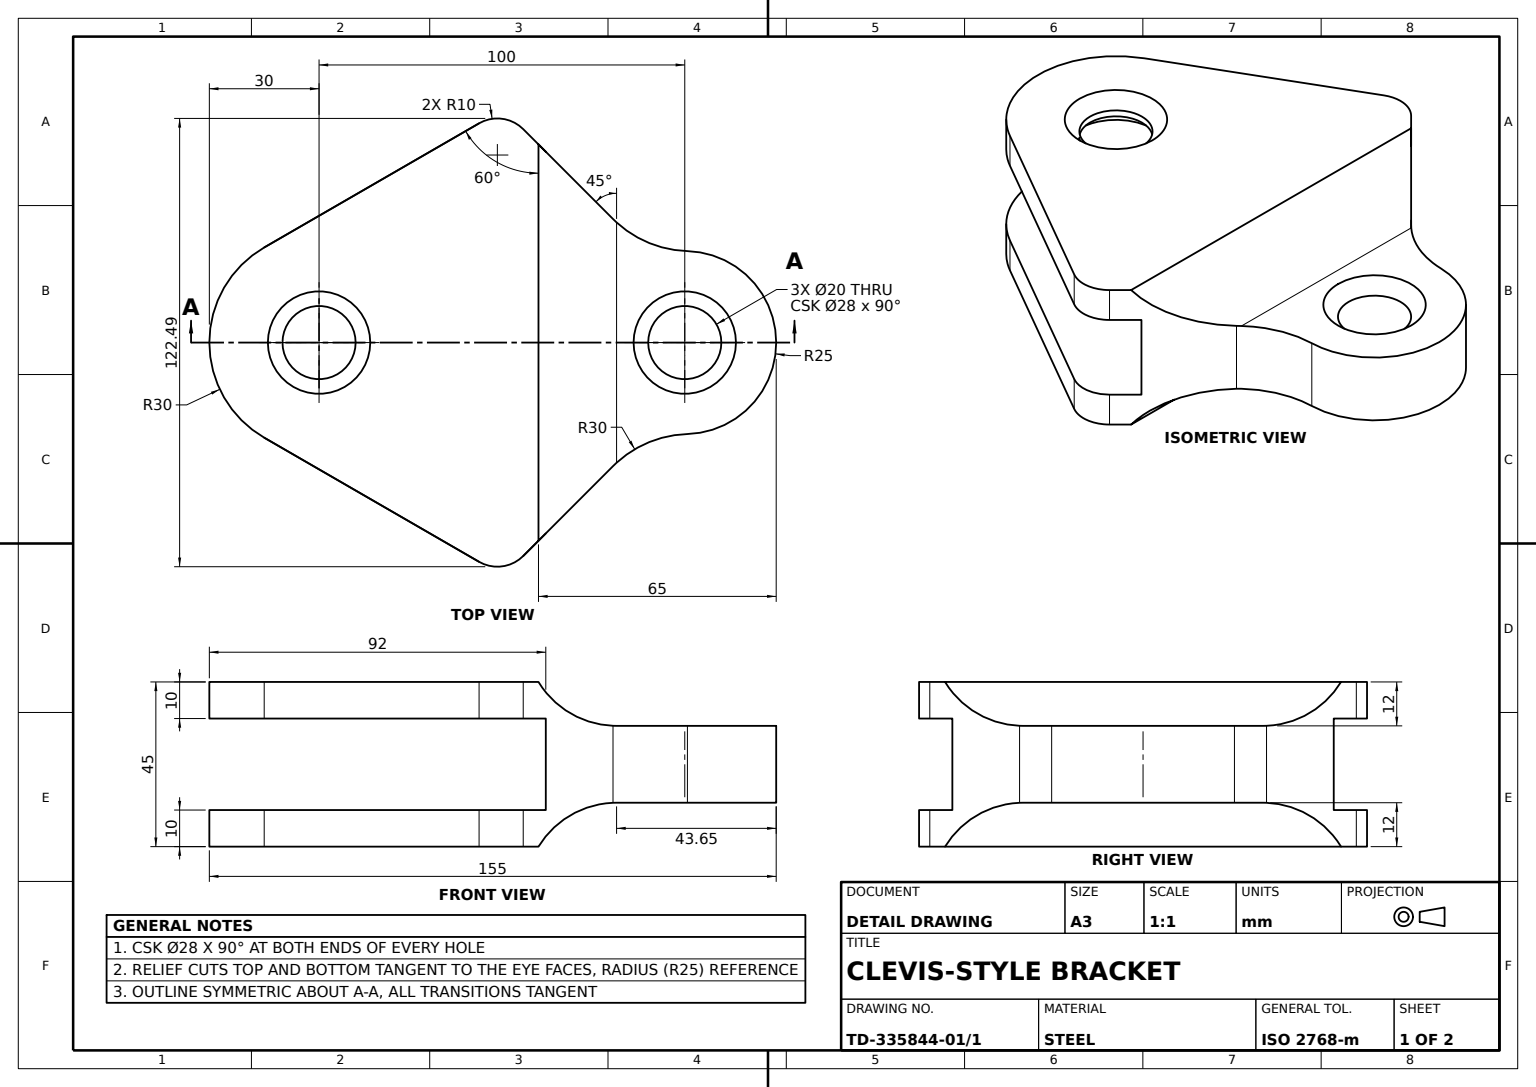
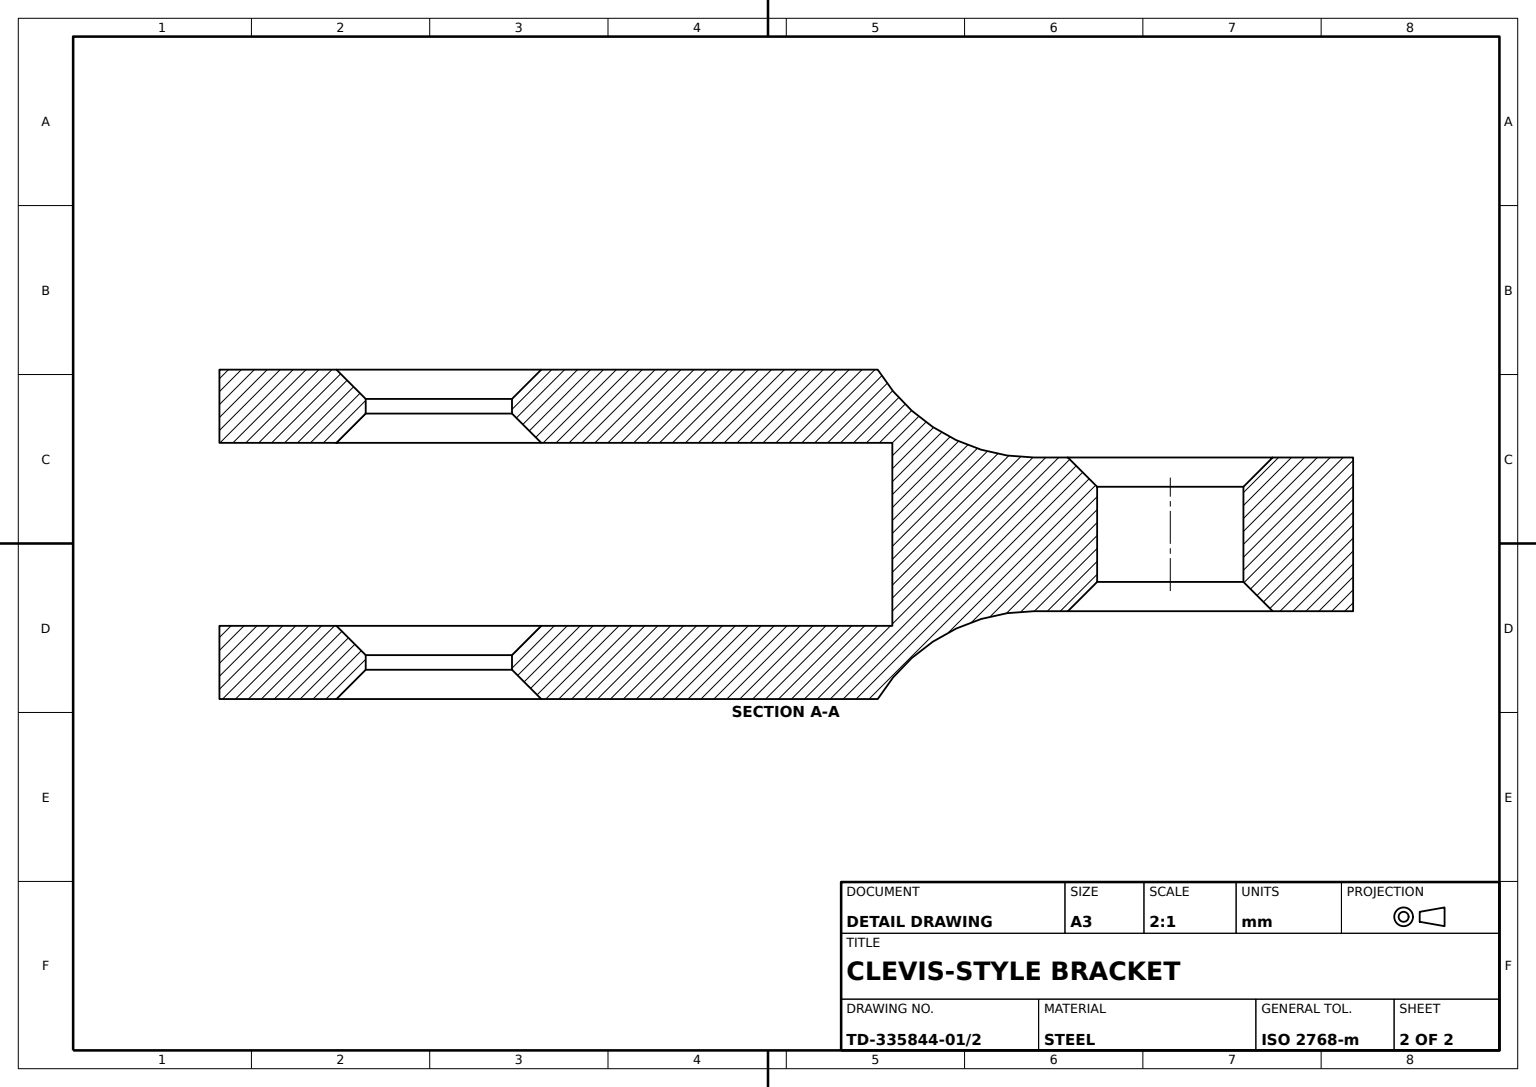
SolidWorks part; units mm, degrees
material "Plain Carbon Steel"
ref_plane "Front Plane" through (0, 0, 0) normal (0, 0, 1) x (1, 0, 0)
ref_plane "Top Plane" through (0, 0, 0) normal (0, 1, 0) x (1, 0, 0)
ref_plane "Right Plane" through (0, 0, 0) normal (1, 0, 0) x (0, 0, -1)
sketch "Bracket Profile Sketch" plane through (0, 0, 0) normal (0, 1, 0) x (1, 0, 0)
  line L0 (0, 0) -> (0, 100) construction
  line L1 (-33.7638, 80.3784) -> (-58.3146, 55.8275)
  line L2 (33.7638, 80.3784) -> (58.3146, 55.8275)
  line L3 (-25.9808, -15) -> (-59.9038, 43.7564)
  line L4 (25.9808, -15) -> (59.9038, 43.7564)
  circle A0 centre (0, 0) radius 10
  arc A1 (-25.9808, -15) -> (25.9808, -15) centre (0, 0) ccw
  circle A2 centre (0, 100) radius 10
  arc A3 (24.9895, 100.7234) -> (-24.9895, 100.7234) centre (0, 100) ccw
  arc A5 (-33.7638, 80.3784) -> (-24.9895, 100.7234) centre (-54.977, 101.5916) ccw
  arc A6 (33.7638, 80.3784) -> (24.9895, 100.7234) centre (54.977, 101.5916) cw
  arc A7 (-58.3146, 55.8275) -> (-59.9038, 43.7564) centre (-51.2436, 48.7564) ccw
  arc A8 (58.3146, 55.8275) -> (59.9038, 43.7564) centre (51.2436, 48.7564) cw
  dimension "D1" = 20
  dimension "D2" = 20
  dimension "D4" = 20
  dimension "D5" = 50
  dimension "D8" = 60
  dimension "D3" = 100
  dimension "D6" = 45
  dimension "D7" = 60
extrude "Bracket Body" add sketch "Bracket Profile Sketch" along normal mid plane 45
ref_plane "Plane1" through (100, 0, 0) normal (1, 0, 0) x (0, 0, -1)
sketch "Clevis Slot Sketch" plane through (100, 0, 0) normal (1, 0, 0) x (0, 0, -1)
  line L0 (-30, 12.5) -> (62, 12.5)
  line L1 (-30, 22.5) -> (-30, -22.5) construction
  line L2 (62, 12.5) -> (62, -12.5)
  line L3 (62, -12.5) -> (-30, -12.5)
  line L5 (-15, 22.5) -> (43.7564, 22.5) construction
  line L7 (-30, 12.5) -> (-30, -12.5)
  dimension "D1" = 25
  dimension "D2" = 10
  dimension "D3" = 92
extrude "Clevis Slot 10mm" cut sketch "Clevis Slot Sketch" against normal blind 375
sketch "Relief Cut Sketch" plane through (100, 0, 0) normal (1, 0, 0) x (0, 0, -1)
  line L0 (60, 22.5) -> (125, 22.5)
  line L4 (81.3542, -10.5) -> (125, -10.5)
  line L5 (125, -22.5) -> (125, 22.5) construction
  line L6 (125, 22.5) -> (125, 10.5)
  line L7 (125, 10.5) -> (81.3542, 10.5)
  line L8 (60, -22.5) -> (125, -22.5)
  line L9 (125, -22.5) -> (125, -10.5)
  arc A0 (81.3542, 10.5) -> (60, 22.5) centre (81.3542, 35.5) cw
  arc A1 (81.3542, -10.5) -> (60, -22.5) centre (81.3542, -35.5) ccw
  point P4 (60, 10.5)
  dimension "D3" = 65
  dimension "D1" = 25
  dimension "D2" = 43.6458
extrude "Relief Cut" cut sketch "Relief Cut Sketch" against normal blind 375
chamfer "Body Edge Chamfer 4mm A" distance 4 1 edges at (0, 22.5, 10)
chamfer "Slot Edge Chamfer 4mm A" distance 4 angle 45 1 edges at (0, 12.5, 10)
chamfer "Body Edge Chamfer 4mm B" distance 4 angle 45 1 edges at (0, -22.5, 10)
chamfer "Slot Edge Chamfer 4mm B" distance 4 angle 45 1 edges at (0, -12.5, -10)
chamfer "Relief Cut Chamfer 4mm" distance 4 angle 45 2 edges at (0, -10.5, -90) (0, 10.5, -110)
